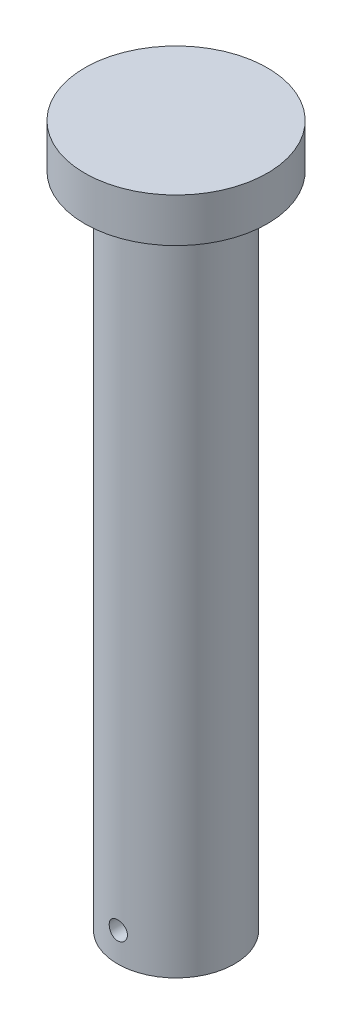
from build123d import *

# Parameters (mm, degrees)
HEAD_PROFILE_SKETCH_R  = 25
HEAD_50X12_DEPTH       = 12
SHANK_PROFILE_SKETCH_R = 16
SHANK_32X180_DEPTH     = 180
CROSS_HOLE_SKETCH_R    = 2.5
CROSS_HOLE_5_DEPTH     = 90


with BuildPart() as part:
    # Head Profile Sketch → Head Ø50x12 (new body)
    with BuildSketch(Plane(origin=(0, 0, 0), x_dir=(1, 0, 0), z_dir=(0, 1, 0))):
        with Locations(Location((0, 0, 0), (0, 0, 270))):
            Circle(HEAD_PROFILE_SKETCH_R)
    extrude(amount=HEAD_50X12_DEPTH)

    # Shank Profile Sketch → Shank Ø32x180 (add)
    with BuildSketch(Plane.XZ):
        with Locations(Location((0, 0, 0), (0, 0, 90))):
            Circle(SHANK_PROFILE_SKETCH_R)
    extrude(amount=SHANK_32X180_DEPTH)

    # Cross Hole Sketch → Cross Hole Ø5 (cut, symmetric)
    with BuildSketch(Plane.XY):
        with Locations(Location((0, -172, 0), (0, 0, 270.000000048))):
            Circle(CROSS_HOLE_SKETCH_R)
    extrude(amount=CROSS_HOLE_5_DEPTH, both=True, mode=Mode.SUBTRACT)


solid = part.part
